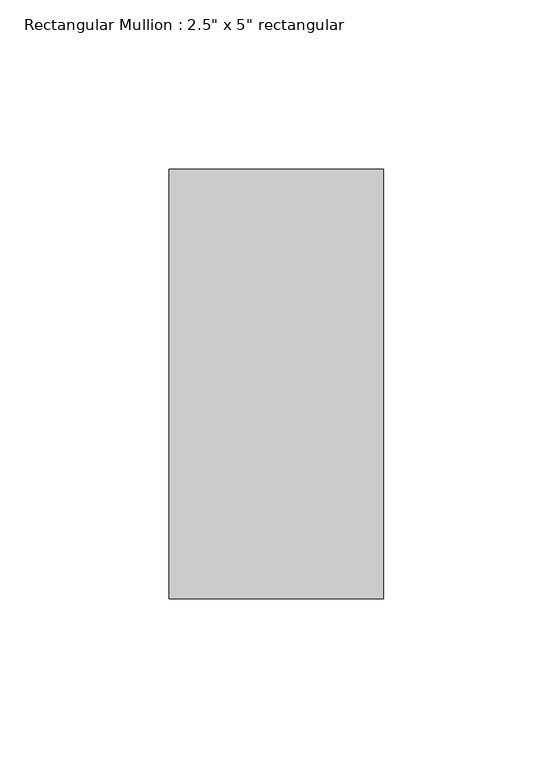
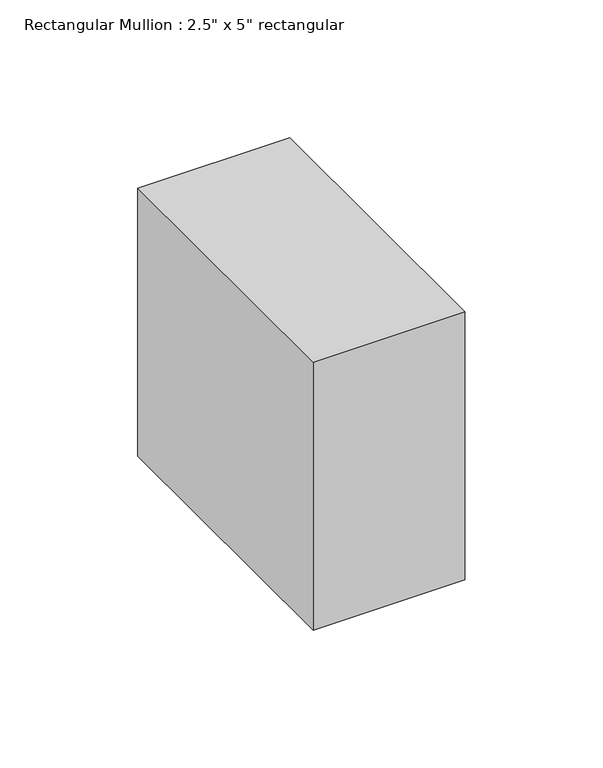
"""IFC4 building model written with IfcOpenShell, lengths in millimetres: member geometry."""

from ifc_helpers import new_model, si_unit, frame, origin, place, context, project, spatial, polyline, outline, extrude, source, transform, mapped, element, save


def member_34b92440(model_context):
    return source(origin(), model_context, "Body", "SweptSolid", [
        extrude(outline(polyline([(31.75, 63.5), (31.75, -63.5), (-31.75, -63.5), (-31.75, 63.5), (31.75, 63.5)])), frame((0.0, 0.0, -118.5333333), z_axis=(0.0, 0.0, 1.0), x_axis=(1.0, 0.0, 0.0)), (0.0, 0.0, 1.0), 118.5333333),
    ])


if __name__ == "__main__":
    model = new_model("IFC4")
    model_context = context("Model", 3, world=origin())
    ifc_project = project(units=[si_unit("LENGTHUNIT", "METRE", prefix="MILLI")], contexts=[model_context])
    site = spatial("IfcSite", under=ifc_project)
    building = spatial("IfcBuilding", under=site)
    placement = place(None, origin())
    member_shape = member_34b92440(model_context)
    element("IfcMember", 1, ObjectType="Rectangular Mullion : 2.5\" x 5\" rectangular", at=placement, inside=building, context=model_context, shape_type="MappedRepresentation", body=[
        mapped(member_shape, transform((0.0, 0.0, 0.0), x_axis=(1.0, 0.0, 0.0), y_axis=(0.0, 1.0, 0.0), z_axis=(0.0, 0.0, 1.0))),
    ])
    save(model, "model.ifc")

# Revit data of these elements
# Type "Rectangular Mullion : 2.5\" x 5\" rectangular"
#   built-in parameter 1007304 = 0.416667 (stored number, unit not read)
#   built-in parameter 1007301 = 0.104167 (stored number, unit not read)
#   built-in parameter 1007300 = 0.104167 (stored number, unit not read)
# Element 1 (IfcMember, "Rectangular Mullion : 2.5\" x 5\" rectangular")
#   Materials on its faces: "Aluminum"
# Materials
#   "Aluminum": class "Metal", colour RGB 247 247 247, transparency 0, Description = "Aluminum 6061", Cost = 0
